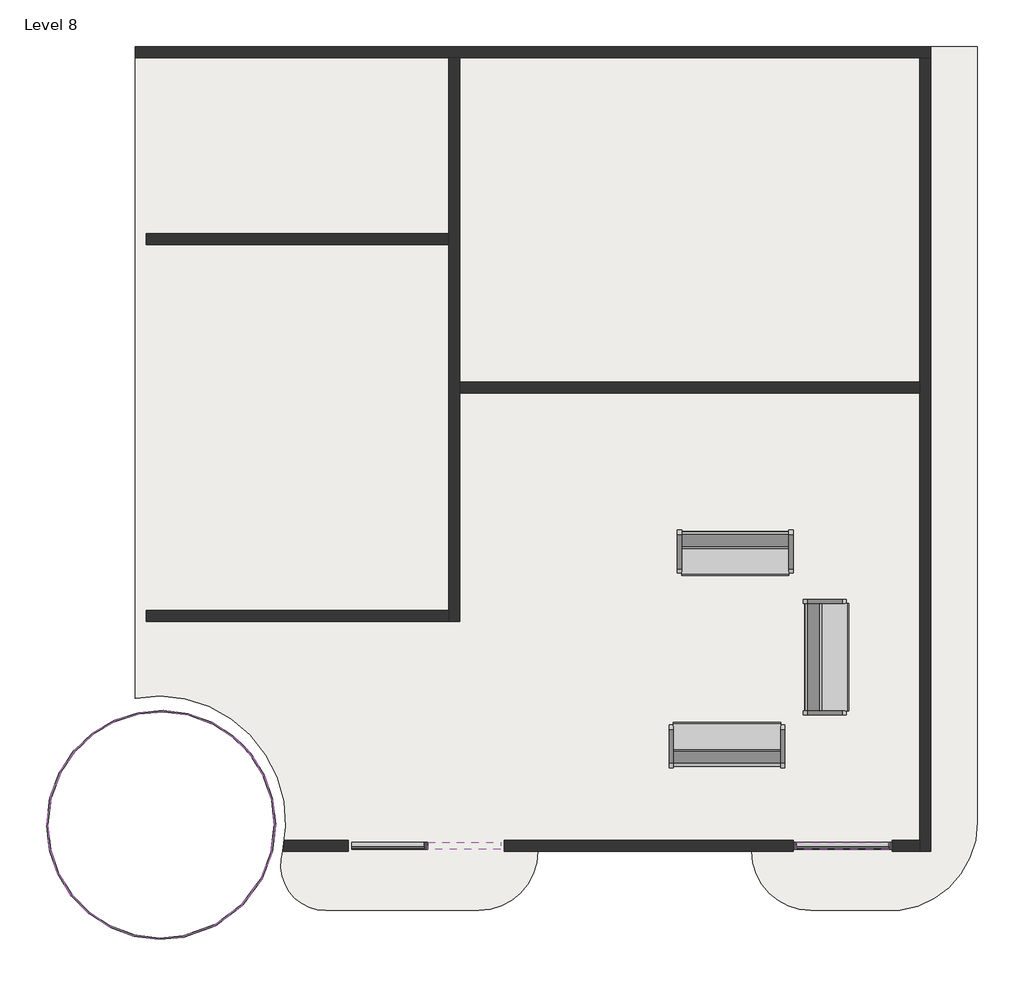
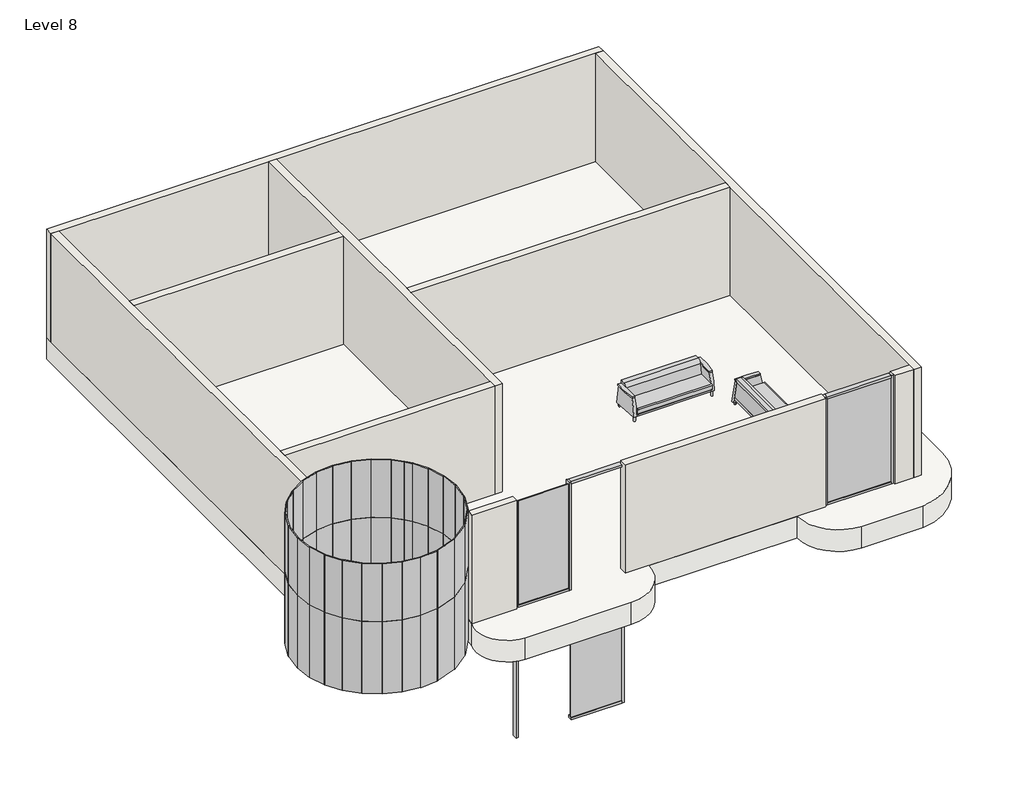
# One storey, incomplete: 59 plates, 11 members, 10 walls, 3 furniture elements, 1 slab.
"""IFC4 building model written with IfcOpenShell, lengths in millimetres."""

from ifc_helpers import new_model, si_unit, point, frame, frame_2d, origin, place, context, project, spatial, polyline, circle_curve, trimmed, segment, composite_curve, outline, extrude, faceted_brep, transform, mapped, element, save
from ifc_brep_helpers import plane_surface, revolved_surface, advanced_brep
from components import furniture_aff9b2fb, member_eaba9652, member_3f395ae9, member_0c868e12, member_7bc42366, system_panel_glazed_f1c144f9, system_panel_glazed_8ed2b2ee, system_panel_glazed_c7815b78, system_panel_glazed_220ba5f3, system_panel_glazed_11fb153e, system_panel_glazed_2f540b85, system_panel_glazed_4848e608, system_panel_glazed_8b35a0ff, system_panel_glazed_87282c25, system_panel_glazed_6d1bb68c, system_panel_glazed_cb3ffd69, system_panel_glazed_404d015f, system_panel_glazed_7b556abe, system_panel_glazed_370bf902

model = new_model("IFC4")

# Units and contexts
model_context = context("Model", 3, world=origin())
ifc_project = project(units=[si_unit("LENGTHUNIT", "METRE", prefix="MILLI")], contexts=[model_context])

# Site, building, storey
site = spatial("IfcSite", under=ifc_project)
building = spatial("IfcBuilding", under=site)
storey = spatial("IfcBuildingStorey", under=building, Name="Level 8", Elevation=21336.0)

# Furniture
placement = place(None, origin())
furniture_shape = furniture_aff9b2fb(model_context)
element("IfcFurniture", 1, ObjectType="Sofa-Pensi : 84\"", at=placement, inside=storey, context=model_context, shape_type="MappedRepresentation", body=[
    mapped(furniture_shape, transform((-2244.8524991, 3650.1964615, 21945.6), x_axis=(1.0, 0.0, 0.0), y_axis=(0.0, 1.0, 0.0), z_axis=(0.0, 0.0, 1.0))),
])
element("IfcFurniture", 2, ObjectType="Sofa-Pensi : 84\"", at=placement, inside=storey, context=model_context, shape_type="MappedRepresentation", body=[
    mapped(furniture_shape, transform((-12.736413, 1720.492712, 21945.6), x_axis=(0.0, 1.0, 0.0), y_axis=(-1.0, 0.0, 0.0), z_axis=(0.0, 0.0, 1.0))),
])
element("IfcFurniture", 3, ObjectType="Sofa-Pensi : 84\"", at=placement, inside=storey, context=model_context, shape_type="MappedRepresentation", body=[
    mapped(furniture_shape, transform((-1840.0399991, 648.4161336, 21945.6), x_axis=(-1.0, 0.0, 0.0), y_axis=(0.0, -1.0, 0.0), z_axis=(0.0, 0.0, 1.0))),
])

# Members
member_shape = member_eaba9652(model_context)
element("IfcMember", 4, ObjectType="Rectangular Mullion : 2.5\" x 5\" rectangular", at=placement, inside=storey, context=model_context, shape_type="MappedRepresentation", body=[
    mapped(member_shape, transform((-7672.5789001, -1482.8937024, 21945.6), x_axis=(-1.0, 0.0, 0.0), y_axis=(0.0, 1.0, 0.0), z_axis=(0.0, 0.0, -1.0))),
])
member_2_shape = member_3f395ae9(model_context)
element("IfcMember", 5, ObjectType="Rectangular Mullion : 2.5\" x 5\" rectangular", at=placement, inside=storey, context=model_context, shape_type="MappedRepresentation", body=[
    mapped(member_2_shape, transform((-9111.7115512, -1482.8937024, 18288.0), x_axis=(-1.0, 0.0, 0.0), y_axis=(0.0, 1.0, 0.0), z_axis=(0.0, 0.0, -1.0))),
])
element("IfcMember", 6, ObjectType="Rectangular Mullion : 2.5\" x 5\" rectangular", at=placement, inside=storey, context=model_context, shape_type="MappedRepresentation", body=[
    mapped(member_2_shape, transform((-899.4462491, -1482.8937024, 21945.6), x_axis=(-1.0, 0.0, 0.0), y_axis=(0.0, 1.0, 0.0), z_axis=(0.0, 0.0, -1.0))),
])
element("IfcMember", 7, ObjectType="Rectangular Mullion : 2.5\" x 5\" rectangular", at=placement, inside=storey, context=model_context, shape_type="MappedRepresentation", body=[
    mapped(member_2_shape, transform((-6233.4462491, -1482.8937024, 21336.0), x_axis=(1.0, 0.0, 0.0), y_axis=(0.0, 1.0, 0.0), z_axis=(0.0, 0.0, 1.0))),
])
element("IfcMember", 8, ObjectType="Rectangular Mullion : 2.5\" x 5\" rectangular", at=placement, inside=storey, context=model_context, shape_type="MappedRepresentation", body=[
    mapped(member_2_shape, transform((929.3537509, -1482.8937024, 24993.6), x_axis=(1.0, 0.0, 0.0), y_axis=(0.0, 1.0, 0.0), z_axis=(0.0, 0.0, 1.0))),
])
member_3_shape = member_0c868e12(model_context)
element("IfcMember", 9, ObjectType="Rectangular Mullion : 2.5\" x 5\" rectangular", at=placement, inside=storey, context=model_context, shape_type="MappedRepresentation", body=[
    mapped(member_3_shape, transform((-9048.2115512, -1482.8937024, 21336.0), x_axis=(0.0, 0.0, 1.0), y_axis=(0.0, 1.0, 0.0), z_axis=(-1.0, 0.0, 0.0))),
])
element("IfcMember", 10, ObjectType="Rectangular Mullion : 2.5\" x 5\" rectangular", at=placement, inside=storey, context=model_context, shape_type="MappedRepresentation", body=[
    mapped(member_3_shape, transform((-7640.8289001, -1482.8937024, 24993.6), x_axis=(0.0, 0.0, 1.0), y_axis=(0.0, 1.0, 0.0), z_axis=(-1.0, 0.0, 0.0))),
])
element("IfcMember", 11, ObjectType="Rectangular Mullion : 2.5\" x 5\" rectangular", at=placement, inside=storey, context=model_context, shape_type="MappedRepresentation", body=[
    mapped(member_3_shape, transform((-6296.9462491, -1482.8937024, 18288.0), x_axis=(0.0, 0.0, -1.0), y_axis=(0.0, 1.0, 0.0), z_axis=(1.0, 0.0, 0.0))),
])
element("IfcMember", 12, ObjectType="Rectangular Mullion : 2.5\" x 5\" rectangular", at=placement, inside=storey, context=model_context, shape_type="MappedRepresentation", body=[
    mapped(member_3_shape, transform((-7704.3289001, -1482.8937024, 21945.6), x_axis=(0.0, 0.0, -1.0), y_axis=(0.0, 1.0, 0.0), z_axis=(1.0, 0.0, 0.0))),
])
member_4_shape = member_7bc42366(model_context)
element("IfcMember", 13, ObjectType="Rectangular Mullion : 2.5\" x 5\" rectangular", at=placement, inside=storey, context=model_context, shape_type="MappedRepresentation", body=[
    mapped(member_4_shape, transform((-835.9462491, -1482.8937024, 24993.6), x_axis=(0.0, 0.0, 1.0), y_axis=(0.0, 1.0, 0.0), z_axis=(-1.0, 0.0, 0.0))),
])
element("IfcMember", 14, ObjectType="Rectangular Mullion : 2.5\" x 5\" rectangular", at=placement, inside=storey, context=model_context, shape_type="MappedRepresentation", body=[
    mapped(member_4_shape, transform((865.8537509, -1482.8937024, 21945.6), x_axis=(0.0, 0.0, -1.0), y_axis=(0.0, 1.0, 0.0), z_axis=(1.0, 0.0, 0.0))),
])

# Plates
system_panel_glazed_shape = system_panel_glazed_f1c144f9(model_context)
element("IfcPlate", 15, ObjectType="System Panel : Glazed", at=placement, inside=storey, context=model_context, shape_type="MappedRepresentation", body=[
    mapped(system_panel_glazed_shape, transform((-14541.9245022, -346.5978939, 21945.6), x_axis=(-0.3551689475306269, -0.9348021281051873, 0.0), y_axis=(0.9348021281051873, -0.3551689475306269, 0.0), z_axis=(0.0, 0.0, 1.0))),
])
element("IfcPlate", 16, ObjectType="System Panel : Glazed", at=placement, inside=storey, context=model_context, shape_type="MappedRepresentation", body=[
    mapped(system_panel_glazed_shape, transform((-10582.1178502, -1851.0877948, 21945.6), x_axis=(0.35516894753064066, 0.934802128105182, 0.0), y_axis=(-0.934802128105182, 0.35516894753064066, 0.0), z_axis=(0.0, 0.0, 1.0))),
])
element("IfcPlate", 17, ObjectType="System Panel : Glazed", at=placement, inside=storey, context=model_context, shape_type="MappedRepresentation", body=[
    mapped(system_panel_glazed_shape, transform((-10459.5232171, -1354.5613954, 21945.6), x_axis=(0.12073632210407237, 0.9926846128175765, 0.0), y_axis=(-0.9926846128175765, 0.12073632210407237, 0.0), z_axis=(0.0, 0.0, 1.0))),
])
element("IfcPlate", 18, ObjectType="System Panel : Glazed", at=placement, inside=storey, context=model_context, shape_type="MappedRepresentation", body=[
    mapped(system_panel_glazed_shape, transform((-14664.5191354, -843.1242933, 21945.6), x_axis=(-0.12073632210406239, -0.9926846128175777, 0.0), y_axis=(0.9926846128175777, -0.12073632210406239, 0.0), z_axis=(0.0, 0.0, 1.0))),
])
system_panel_glazed_2_shape = system_panel_glazed_8ed2b2ee(model_context)
element("IfcPlate", 19, ObjectType="System Panel : Glazed", at=placement, inside=storey, context=model_context, shape_type="MappedRepresentation", body=[
    mapped(system_panel_glazed_2_shape, transform((-11841.3777431, -3082.3793017, 21945.6), x_axis=(0.9398911711666007, 0.3414741371803665, 0.0), y_axis=(-0.3414741371803665, 0.9398911711666007, 0.0), z_axis=(0.0, 0.0, 1.0))),
])
element("IfcPlate", 20, ObjectType="System Panel : Glazed", at=placement, inside=storey, context=model_context, shape_type="MappedRepresentation", body=[
    mapped(system_panel_glazed_2_shape, transform((-10858.9635423, -2345.1728692, 21945.6), x_axis=(0.5905687200141164, 0.8069873524045393, 0.0), y_axis=(-0.8069873524045393, 0.5905687200141164, 0.0), z_axis=(0.0, 0.0, 1.0))),
])
element("IfcPlate", 21, ObjectType="System Panel : Glazed", at=placement, inside=storey, context=model_context, shape_type="MappedRepresentation", body=[
    mapped(system_panel_glazed_2_shape, transform((-11295.3522982, -2786.8279712, 21945.6), x_axis=(0.7998453025525061, 0.6002062078858317, 0.0), y_axis=(-0.6002062078858317, 0.7998453025525061, 0.0), z_axis=(0.0, 0.0, 1.0))),
])
system_panel_glazed_3_shape = system_panel_glazed_c7815b78(model_context)
element("IfcPlate", 22, ObjectType="System Panel : Glazed", at=placement, inside=storey, context=model_context, shape_type="MappedRepresentation", body=[
    mapped(system_panel_glazed_3_shape, transform((-10454.4737362, -864.5204039, 21945.6), x_axis=(-0.11050163420416614, 0.993875942378227, 0.0), y_axis=(-0.993875942378227, -0.11050163420416614, 0.0), z_axis=(0.0, 0.0, 1.0))),
])
element("IfcPlate", 23, ObjectType="System Panel : Glazed", at=placement, inside=storey, context=model_context, shape_type="MappedRepresentation", body=[
    mapped(system_panel_glazed_3_shape, transform((-14669.5686163, -1333.1652848, 21945.6), x_axis=(0.11050163420415136, -0.9938759423782286, 0.0), y_axis=(0.9938759423782286, 0.11050163420415136, 0.0), z_axis=(0.0, 0.0, 1.0))),
])
element("IfcPlate", 24, ObjectType="System Panel : Glazed", at=placement, inside=storey, context=model_context, shape_type="MappedRepresentation", body=[
    mapped(system_panel_glazed_3_shape, transform((-11410.1424167, 681.5611944, 21945.6), x_axis=(-0.8396018558176894, 0.5432022861766066, 0.0), y_axis=(-0.5432022861766066, -0.8396018558176894, 0.0), z_axis=(0.0, 0.0, 1.0))),
])
element("IfcPlate", 25, ObjectType="System Panel : Glazed", at=placement, inside=storey, context=model_context, shape_type="MappedRepresentation", body=[
    mapped(system_panel_glazed_3_shape, transform((-13212.0893695, 919.590846, 21945.6), x_axis=(-0.9518517343814786, -0.3065587639506839, 0.0), y_axis=(0.3065587639506839, -0.9518517343814786, 0.0), z_axis=(0.0, 0.0, 1.0))),
])
element("IfcPlate", 26, ObjectType="System Panel : Glazed", at=placement, inside=storey, context=model_context, shape_type="MappedRepresentation", body=[
    mapped(system_panel_glazed_3_shape, transform((-12839.7224363, -3201.1142893, 21945.6), x_axis=(0.9913878918151698, -0.1309581916577702, 0.0), y_axis=(0.1309581916577702, 0.9913878918151698, 0.0), z_axis=(0.0, 0.0, 1.0))),
])
element("IfcPlate", 27, ObjectType="System Panel : Glazed", at=placement, inside=storey, context=model_context, shape_type="MappedRepresentation", body=[
    mapped(system_panel_glazed_3_shape, transform((-14365.783041, -2213.7896382, 21945.6), x_axis=(0.5257859322352114, -0.8506169252157811, 0.0), y_axis=(0.8506169252157811, 0.5257859322352114, 0.0), z_axis=(0.0, 0.0, 1.0))),
])
element("IfcPlate", 28, ObjectType="System Panel : Glazed", at=placement, inside=storey, context=model_context, shape_type="MappedRepresentation", body=[
    mapped(system_panel_glazed_3_shape, transform((-13713.8999358, -2879.2468831, 21945.6), x_axis=(0.8396018558176805, -0.5432022861766201, 0.0), y_axis=(0.5432022861766201, 0.8396018558176805, 0.0), z_axis=(0.0, 0.0, 1.0))),
])
element("IfcPlate", 29, ObjectType="System Panel : Glazed", at=placement, inside=storey, context=model_context, shape_type="MappedRepresentation", body=[
    mapped(system_panel_glazed_3_shape, transform((-14014.4059364, 446.2272921, 21945.6), x_axis=(-0.7286232370002992, -0.6849147235263715, 0.0), y_axis=(0.6849147235263715, -0.7286232370002992, 0.0), z_axis=(0.0, 0.0, 1.0))),
])
element("IfcPlate", 30, ObjectType="System Panel : Glazed", at=placement, inside=storey, context=model_context, shape_type="MappedRepresentation", body=[
    mapped(system_panel_glazed_3_shape, transform((-12284.3199161, 1003.4286006, 21945.6), x_axis=(-0.9913878918151723, 0.13095819165775144, 0.0), y_axis=(-0.13095819165775144, -0.9913878918151723, 0.0), z_axis=(0.0, 0.0, 1.0))),
])
element("IfcPlate", 31, ObjectType="System Panel : Glazed", at=placement, inside=storey, context=model_context, shape_type="MappedRepresentation", body=[
    mapped(system_panel_glazed_3_shape, transform((-12752.8652893, 1013.0855973, 21945.6), x_axis=(-0.9959419324521102, -0.08999815100076568, 0.0), y_axis=(0.08999815100076568, -0.9959419324521102, 0.0), z_axis=(0.0, 0.0, 1.0))),
])
element("IfcPlate", 32, ObjectType="System Panel : Glazed", at=placement, inside=storey, context=model_context, shape_type="MappedRepresentation", body=[
    mapped(system_panel_glazed_3_shape, transform((-11829.3381514, 891.0915272, 21945.6), x_axis=(-0.9384120429483949, 0.3455182160891376, 0.0), y_axis=(-0.3455182160891376, -0.9384120429483949, 0.0), z_axis=(0.0, 0.0, 1.0))),
])
element("IfcPlate", 33, ObjectType="System Panel : Glazed", at=placement, inside=storey, context=model_context, shape_type="MappedRepresentation", body=[
    mapped(system_panel_glazed_3_shape, transform((-10557.4115054, -407.3204039, 21945.6), x_axis=(-0.3261077326604367, 0.9453326116764772, 0.0), y_axis=(-0.9453326116764772, -0.3261077326604367, 0.0), z_axis=(0.0, 0.0, 1.0))),
])
element("IfcPlate", 34, ObjectType="System Panel : Glazed", at=placement, inside=storey, context=model_context, shape_type="MappedRepresentation", body=[
    mapped(system_panel_glazed_3_shape, transform((-12371.1770631, -3210.771286, 21945.6), x_axis=(0.9959419324521115, 0.08999815100075001, 0.0), y_axis=(-0.08999815100075001, 0.9959419324521115, 0.0), z_axis=(0.0, 0.0, 1.0))),
])
element("IfcPlate", 35, ObjectType="System Panel : Glazed", at=placement, inside=storey, context=model_context, shape_type="MappedRepresentation", body=[
    mapped(system_panel_glazed_3_shape, transform((-13294.7042011, -3088.7772159, 21945.6), x_axis=(0.9384120429483891, -0.34551821608915334, 0.0), y_axis=(0.34551821608915334, 0.9384120429483891, 0.0), z_axis=(0.0, 0.0, 1.0))),
])
element("IfcPlate", 36, ObjectType="System Panel : Glazed", at=placement, inside=storey, context=model_context, shape_type="MappedRepresentation", body=[
    mapped(system_panel_glazed_3_shape, transform((-14076.8350959, -2582.7572647, 21945.6), x_axis=(0.6997834615185511, -0.7143550286692988, 0.0), y_axis=(0.7143550286692988, 0.6997834615185511, 0.0), z_axis=(0.0, 0.0, 1.0))),
])
element("IfcPlate", 37, ObjectType="System Panel : Glazed", at=placement, inside=storey, context=model_context, shape_type="MappedRepresentation", body=[
    mapped(system_panel_glazed_3_shape, transform((-14566.6308471, -1790.3652848, 21945.6), x_axis=(0.32610773266042153, -0.9453326116764824, 0.0), y_axis=(0.9453326116764824, 0.32610773266042153, 0.0), z_axis=(0.0, 0.0, 1.0))),
])
element("IfcPlate", 38, ObjectType="System Panel : Glazed", at=placement, inside=storey, context=model_context, shape_type="MappedRepresentation", body=[
    mapped(system_panel_glazed_3_shape, transform((-14318.3113206, 89.4787227, 21945.6), x_axis=(-0.5603879632167612, -0.8282302401396425, 0.0), y_axis=(0.8282302401396425, -0.5603879632167612, 0.0), z_axis=(0.0, 0.0, 1.0))),
])
element("IfcPlate", 39, ObjectType="System Panel : Glazed", at=placement, inside=storey, context=model_context, shape_type="MappedRepresentation", body=[
    mapped(system_panel_glazed_3_shape, transform((-13639.5625299, 727.5108588, 21945.6), x_axis=(-0.8612707706620224, -0.5081462974412448, 0.0), y_axis=(0.5081462974412448, -0.8612707706620224, 0.0), z_axis=(0.0, 0.0, 1.0))),
])
system_panel_glazed_4_shape = system_panel_glazed_220ba5f3(model_context)
element("IfcPlate", 40, ObjectType="System Panel : Glazed", at=placement, inside=storey, context=model_context, shape_type="MappedRepresentation", body=[
    mapped(system_panel_glazed_4_shape, transform((-10742.3305673, -4.7597883, 21945.6), x_axis=(-0.5152811917631037, 0.8570211744263939, 0.0), y_axis=(-0.8570211744263939, -0.5152811917631037, 0.0), z_axis=(0.0, 0.0, 1.0))),
])
system_panel_glazed_5_shape = system_panel_glazed_11fb153e(model_context)
element("IfcPlate", 41, ObjectType="System Panel : Glazed", at=placement, inside=storey, context=model_context, shape_type="MappedRepresentation", body=[
    mapped(system_panel_glazed_5_shape, transform((-11098.0043985, 445.2241463, 21945.6), x_axis=(-0.7256671855033587, 0.6880458821064435, 0.0), y_axis=(-0.6880458821064435, -0.7256671855033587, 0.0), z_axis=(0.0, 0.0, 1.0))),
])
system_panel_glazed_6_shape = system_panel_glazed_2f540b85(model_context)
element("IfcPlate", 42, ObjectType="System Panel : Glazed", at=placement, inside=storey, context=model_context, shape_type="MappedRepresentation", body=[
    mapped(system_panel_glazed_6_shape, transform((-10917.0903061, 255.9395759, 21945.6), x_axis=(-0.6357445726375757, 0.7718995001694627, 0.0), y_axis=(-0.7718995001694627, -0.6357445726375757, 0.0), z_axis=(0.0, 0.0, 1.0))),
])
system_panel_glazed_7_shape = system_panel_glazed_4848e608(model_context)
element("IfcPlate", 43, ObjectType="System Panel : Glazed", at=placement, inside=storey, context=model_context, shape_type="MappedRepresentation", body=[
    mapped(system_panel_glazed_7_shape, transform((-14669.5686163, -1333.1652848, 23977.6), x_axis=(0.11050163420415136, -0.9938759423782286, 0.0), y_axis=(0.9938759423782286, 0.11050163420415136, 0.0), z_axis=(0.0, 0.0, 1.0))),
])
element("IfcPlate", 44, ObjectType="System Panel : Glazed", at=placement, inside=storey, context=model_context, shape_type="MappedRepresentation", body=[
    mapped(system_panel_glazed_7_shape, transform((-14365.783041, -2213.7896382, 23977.6), x_axis=(0.5257859322352114, -0.8506169252157811, 0.0), y_axis=(0.8506169252157811, 0.5257859322352114, 0.0), z_axis=(0.0, 0.0, 1.0))),
])
element("IfcPlate", 45, ObjectType="System Panel : Glazed", at=placement, inside=storey, context=model_context, shape_type="MappedRepresentation", body=[
    mapped(system_panel_glazed_7_shape, transform((-13713.8999358, -2879.2468831, 23977.6), x_axis=(0.8396018558176805, -0.5432022861766201, 0.0), y_axis=(0.5432022861766201, 0.8396018558176805, 0.0), z_axis=(0.0, 0.0, 1.0))),
])
element("IfcPlate", 46, ObjectType="System Panel : Glazed", at=placement, inside=storey, context=model_context, shape_type="MappedRepresentation", body=[
    mapped(system_panel_glazed_7_shape, transform((-12839.7224363, -3201.1142893, 23977.6), x_axis=(0.9913878918151698, -0.13095819165777017, 0.0), y_axis=(0.13095819165777017, 0.9913878918151698, 0.0), z_axis=(0.0, 0.0, 1.0))),
])
element("IfcPlate", 47, ObjectType="System Panel : Glazed", at=placement, inside=storey, context=model_context, shape_type="MappedRepresentation", body=[
    mapped(system_panel_glazed_7_shape, transform((-12371.1770631, -3210.771286, 23977.6), x_axis=(0.9959419324521115, 0.08999815100075001, 0.0), y_axis=(-0.08999815100075001, 0.9959419324521115, 0.0), z_axis=(0.0, 0.0, 1.0))),
])
element("IfcPlate", 48, ObjectType="System Panel : Glazed", at=placement, inside=storey, context=model_context, shape_type="MappedRepresentation", body=[
    mapped(system_panel_glazed_7_shape, transform((-13294.7042011, -3088.7772159, 23977.6), x_axis=(0.9384120429483891, -0.34551821608915334, 0.0), y_axis=(0.34551821608915334, 0.9384120429483891, 0.0), z_axis=(0.0, 0.0, 1.0))),
])
element("IfcPlate", 49, ObjectType="System Panel : Glazed", at=placement, inside=storey, context=model_context, shape_type="MappedRepresentation", body=[
    mapped(system_panel_glazed_7_shape, transform((-14076.8350959, -2582.7572647, 23977.6), x_axis=(0.6997834615185511, -0.7143550286692988, 0.0), y_axis=(0.7143550286692988, 0.6997834615185511, 0.0), z_axis=(0.0, 0.0, 1.0))),
])
element("IfcPlate", 50, ObjectType="System Panel : Glazed", at=placement, inside=storey, context=model_context, shape_type="MappedRepresentation", body=[
    mapped(system_panel_glazed_7_shape, transform((-14566.6308471, -1790.3652848, 23977.6), x_axis=(0.32610773266042153, -0.9453326116764824, 0.0), y_axis=(0.9453326116764824, 0.32610773266042153, 0.0), z_axis=(0.0, 0.0, 1.0))),
])
element("IfcPlate", 51, ObjectType="System Panel : Glazed", at=placement, inside=storey, context=model_context, shape_type="MappedRepresentation", body=[
    mapped(system_panel_glazed_7_shape, transform((-10454.4737362, -864.5204039, 23977.6), x_axis=(-0.11050163420416614, 0.993875942378227, 0.0), y_axis=(-0.993875942378227, -0.11050163420416614, 0.0), z_axis=(0.0, 0.0, 1.0))),
])
element("IfcPlate", 52, ObjectType="System Panel : Glazed", at=placement, inside=storey, context=model_context, shape_type="MappedRepresentation", body=[
    mapped(system_panel_glazed_7_shape, transform((-10557.4115054, -407.3204039, 23977.6), x_axis=(-0.3261077326604368, 0.9453326116764772, 0.0), y_axis=(-0.9453326116764772, -0.3261077326604368, 0.0), z_axis=(0.0, 0.0, 1.0))),
])
element("IfcPlate", 53, ObjectType="System Panel : Glazed", at=placement, inside=storey, context=model_context, shape_type="MappedRepresentation", body=[
    mapped(system_panel_glazed_7_shape, transform((-11410.1424167, 681.5611944, 23977.6), x_axis=(-0.8396018558176894, 0.5432022861766066, 0.0), y_axis=(-0.5432022861766066, -0.8396018558176894, 0.0), z_axis=(0.0, 0.0, 1.0))),
])
element("IfcPlate", 54, ObjectType="System Panel : Glazed", at=placement, inside=storey, context=model_context, shape_type="MappedRepresentation", body=[
    mapped(system_panel_glazed_7_shape, transform((-11829.3381514, 891.0915272, 23977.6), x_axis=(-0.9384120429483949, 0.3455182160891376, 0.0), y_axis=(-0.3455182160891376, -0.9384120429483949, 0.0), z_axis=(0.0, 0.0, 1.0))),
])
element("IfcPlate", 55, ObjectType="System Panel : Glazed", at=placement, inside=storey, context=model_context, shape_type="MappedRepresentation", body=[
    mapped(system_panel_glazed_7_shape, transform((-12284.3199161, 1003.4286006, 23977.6), x_axis=(-0.9913878918151723, 0.1309581916577514, 0.0), y_axis=(-0.1309581916577514, -0.9913878918151723, 0.0), z_axis=(0.0, 0.0, 1.0))),
])
element("IfcPlate", 56, ObjectType="System Panel : Glazed", at=placement, inside=storey, context=model_context, shape_type="MappedRepresentation", body=[
    mapped(system_panel_glazed_7_shape, transform((-12752.8652893, 1013.0855973, 23977.6), x_axis=(-0.9959419324521102, -0.08999815100076568, 0.0), y_axis=(0.08999815100076568, -0.9959419324521102, 0.0), z_axis=(0.0, 0.0, 1.0))),
])
element("IfcPlate", 57, ObjectType="System Panel : Glazed", at=placement, inside=storey, context=model_context, shape_type="MappedRepresentation", body=[
    mapped(system_panel_glazed_7_shape, transform((-13212.0893695, 919.590846, 23977.6), x_axis=(-0.9518517343814786, -0.3065587639506839, 0.0), y_axis=(0.3065587639506839, -0.9518517343814786, 0.0), z_axis=(0.0, 0.0, 1.0))),
])
element("IfcPlate", 58, ObjectType="System Panel : Glazed", at=placement, inside=storey, context=model_context, shape_type="MappedRepresentation", body=[
    mapped(system_panel_glazed_7_shape, transform((-13639.5625299, 727.5108588, 23977.6), x_axis=(-0.8612707706620223, -0.508146297441245, 0.0), y_axis=(0.508146297441245, -0.8612707706620223, 0.0), z_axis=(0.0, 0.0, 1.0))),
])
element("IfcPlate", 59, ObjectType="System Panel : Glazed", at=placement, inside=storey, context=model_context, shape_type="MappedRepresentation", body=[
    mapped(system_panel_glazed_7_shape, transform((-14014.4059364, 446.2272921, 23977.6), x_axis=(-0.7286232370002992, -0.6849147235263715, 0.0), y_axis=(0.6849147235263715, -0.7286232370002992, 0.0), z_axis=(0.0, 0.0, 1.0))),
])
element("IfcPlate", 60, ObjectType="System Panel : Glazed", at=placement, inside=storey, context=model_context, shape_type="MappedRepresentation", body=[
    mapped(system_panel_glazed_7_shape, transform((-14318.3113206, 89.4787227, 23977.6), x_axis=(-0.5603879632167612, -0.8282302401396425, 0.0), y_axis=(0.8282302401396425, -0.5603879632167612, 0.0), z_axis=(0.0, 0.0, 1.0))),
])
system_panel_glazed_8_shape = system_panel_glazed_8b35a0ff(model_context)
element("IfcPlate", 61, ObjectType="System Panel : Glazed", at=placement, inside=storey, context=model_context, shape_type="MappedRepresentation", body=[
    mapped(system_panel_glazed_8_shape, transform((-10742.3305673, -4.7597883, 23977.6), x_axis=(-0.5152811917631037, 0.8570211744263939, 0.0), y_axis=(-0.8570211744263939, -0.5152811917631037, 0.0), z_axis=(0.0, 0.0, 1.0))),
])
system_panel_glazed_9_shape = system_panel_glazed_87282c25(model_context)
element("IfcPlate", 62, ObjectType="System Panel : Glazed", at=placement, inside=storey, context=model_context, shape_type="MappedRepresentation", body=[
    mapped(system_panel_glazed_9_shape, transform((-10917.0903061, 255.9395759, 23977.6), x_axis=(-0.6357445726375757, 0.7718995001694627, 0.0), y_axis=(-0.7718995001694627, -0.6357445726375757, 0.0), z_axis=(0.0, 0.0, 1.0))),
])
system_panel_glazed_10_shape = system_panel_glazed_6d1bb68c(model_context)
element("IfcPlate", 63, ObjectType="System Panel : Glazed", at=placement, inside=storey, context=model_context, shape_type="MappedRepresentation", body=[
    mapped(system_panel_glazed_10_shape, transform((-11098.0043985, 445.2241463, 23977.6), x_axis=(-0.7256671855033587, 0.6880458821064435, 0.0), y_axis=(-0.6880458821064435, -0.7256671855033587, 0.0), z_axis=(0.0, 0.0, 1.0))),
])
system_panel_glazed_11_shape = system_panel_glazed_cb3ffd69(model_context)
element("IfcPlate", 64, ObjectType="System Panel : Glazed", at=placement, inside=storey, context=model_context, shape_type="MappedRepresentation", body=[
    mapped(system_panel_glazed_11_shape, transform((-10582.1178502, -1851.0877948, 23977.6), x_axis=(0.35516894753064066, 0.934802128105182, 0.0), y_axis=(-0.934802128105182, 0.35516894753064066, 0.0), z_axis=(0.0, 0.0, 1.0))),
])
element("IfcPlate", 65, ObjectType="System Panel : Glazed", at=placement, inside=storey, context=model_context, shape_type="MappedRepresentation", body=[
    mapped(system_panel_glazed_11_shape, transform((-10459.5232171, -1354.5613954, 23977.6), x_axis=(0.1207363221040724, 0.9926846128175765, 0.0), y_axis=(-0.9926846128175765, 0.1207363221040724, 0.0), z_axis=(0.0, 0.0, 1.0))),
])
element("IfcPlate", 66, ObjectType="System Panel : Glazed", at=placement, inside=storey, context=model_context, shape_type="MappedRepresentation", body=[
    mapped(system_panel_glazed_11_shape, transform((-14541.9245022, -346.5978939, 23977.6), x_axis=(-0.3551689475306269, -0.9348021281051873, 0.0), y_axis=(0.9348021281051873, -0.3551689475306269, 0.0), z_axis=(0.0, 0.0, 1.0))),
])
element("IfcPlate", 67, ObjectType="System Panel : Glazed", at=placement, inside=storey, context=model_context, shape_type="MappedRepresentation", body=[
    mapped(system_panel_glazed_11_shape, transform((-14664.5191354, -843.1242933, 23977.6), x_axis=(-0.1207363221040624, -0.9926846128175777, 0.0), y_axis=(0.9926846128175777, -0.1207363221040624, 0.0), z_axis=(0.0, 0.0, 1.0))),
])
system_panel_glazed_12_shape = system_panel_glazed_404d015f(model_context)
element("IfcPlate", 68, ObjectType="System Panel : Glazed", at=placement, inside=storey, context=model_context, shape_type="MappedRepresentation", body=[
    mapped(system_panel_glazed_12_shape, transform((-11841.3777431, -3082.3793017, 23977.6), x_axis=(0.9398911711666007, 0.3414741371803665, 0.0), y_axis=(-0.3414741371803665, 0.9398911711666007, 0.0), z_axis=(0.0, 0.0, 1.0))),
])
element("IfcPlate", 69, ObjectType="System Panel : Glazed", at=placement, inside=storey, context=model_context, shape_type="MappedRepresentation", body=[
    mapped(system_panel_glazed_12_shape, transform((-10858.9635423, -2345.1728692, 23977.6), x_axis=(0.5905687200141164, 0.8069873524045393, 0.0), y_axis=(-0.8069873524045393, 0.5905687200141164, 0.0), z_axis=(0.0, 0.0, 1.0))),
])
element("IfcPlate", 70, ObjectType="System Panel : Glazed", at=placement, inside=storey, context=model_context, shape_type="MappedRepresentation", body=[
    mapped(system_panel_glazed_12_shape, transform((-11295.3522982, -2786.8279712, 23977.6), x_axis=(0.7998453025525062, 0.6002062078858316, 0.0), y_axis=(-0.6002062078858316, 0.7998453025525062, 0.0), z_axis=(0.0, 0.0, 1.0))),
])
system_panel_glazed_13_shape = system_panel_glazed_7b556abe(model_context)
element("IfcPlate", 71, ObjectType="System Panel : Glazed", at=placement, inside=storey, context=model_context, shape_type="MappedRepresentation", body=[
    mapped(system_panel_glazed_13_shape, transform((-6968.8875746, -1482.8937024, 18351.5), x_axis=(-1.0, 0.0, 0.0), y_axis=(0.0, -1.0, 0.0), z_axis=(0.0, 0.0, 1.0))),
])
element("IfcPlate", 72, ObjectType="System Panel : Glazed", at=placement, inside=storey, context=model_context, shape_type="MappedRepresentation", body=[
    mapped(system_panel_glazed_13_shape, transform((-8376.2702257, -1482.8937024, 22009.1), x_axis=(-1.0, 0.0, 0.0), y_axis=(0.0, -1.0, 0.0), z_axis=(0.0, 0.0, 1.0))),
])
system_panel_glazed_14_shape = system_panel_glazed_370bf902(model_context)
element("IfcPlate", 73, ObjectType="System Panel : Glazed", at=placement, inside=storey, context=model_context, shape_type="MappedRepresentation", body=[
    mapped(system_panel_glazed_14_shape, transform((14.9537509, -1482.8937024, 22009.1), x_axis=(-1.0, 0.0, 0.0), y_axis=(0.0, -1.0, 0.0), z_axis=(0.0, 0.0, 1.0))),
])

# Slab
element("IfcSlab", 74, ObjectType="Generic - 2'", at=placement, inside=storey, context=model_context, shape_type="SweptSolid", body=[
    extrude(outline(composite_curve([segment(polyline([(2504.1537509, 13274.5062976), (2504.1537509, -1051.0937024)]), True, "CONTINUOUS"), segment(trimmed(circle_curve(frame_2d((865.9099456, -1051.0937024)), 1638.2438053), [point((2504.1537509, -1051.0937024))], [point((1069.0537509, -2676.6937024))], False, "CARTESIAN"), True, "CONTINUOUS"), segment(polyline([(1069.0537509, -2676.6937024), (-569.2462491, -2676.6937024)]), True, "CONTINUOUS"), segment(trimmed(circle_curve(frame_2d((-569.2462491, -1584.4937024)), 1092.2), [point((-569.2462491, -2676.6937024))], [point((-1661.4462491, -1584.4937024))], False, "CARTESIAN"), True, "CONTINUOUS"), segment(polyline([(-1661.4462491, -1584.4937024), (-5609.8647377, -1584.4937024)]), True, "CONTINUOUS"), segment(trimmed(circle_curve(frame_2d((-6702.0647377, -1584.4937024)), 1092.2), [point((-5609.8647377, -1584.4937024))], [point((-6702.0647377, -2676.6937024))], False, "CARTESIAN"), True, "CONTINUOUS"), segment(polyline([(-6702.0647377, -2676.6937024), (-9521.4647377, -2676.6937024)]), True, "CONTINUOUS"), segment(trimmed(circle_curve(frame_2d((-9521.4647377, -1843.8920375)), 832.801665), [point((-9521.4647377, -2676.6937024))], [point((-10312.8376694, -1584.4937024))], False, "CARTESIAN"), True, "CONTINUOUS"), segment(trimmed(circle_curve(frame_2d((-12612.6150686, -1075.1054509)), 2355.5153315), [point((-10312.8376694, -1584.4937024))], [point((-13040.6462491, 1241.1937063))], True, "CARTESIAN"), True, "CONTINUOUS"), segment(polyline([(-13040.6462491, 1241.1937063), (-13040.6462491, 13274.5062976), (2504.1537509, 13274.5062976)]), True, "CONTINUOUS")], self_intersect=False)), frame((0.0, 0.0, 21336.0), z_axis=(0.0, 0.0, 1.0), x_axis=(1.0, 0.0, 0.0)), (0.0, 0.0, 1.0), 609.6),
])

# Walls
element("IfcWall", 75, ObjectType="Generic - 8\"", at=placement, inside=storey, context=model_context, shape_type="Brep", body=[
    faceted_brep([(-13040.6462491, 13071.3062976, 21945.6), (-12837.4462491, 13071.3062976, 21945.6), (-7249.4462491, 13071.3062976, 21945.6), (-7046.2462491, 13071.3062976, 21945.6), (1437.3537509, 13071.3062976, 21945.6), (1640.5537509, 13071.3062976, 21945.6), (1640.5537509, 13071.3062976, 24993.6), (1437.3537509, 13071.3062976, 24993.6), (-7046.2462491, 13071.3062976, 24993.6), (-7249.4462491, 13071.3062976, 24993.6), (-12837.4462491, 13071.3062976, 24993.6), (-13040.6462491, 13071.3062976, 24993.6), (-13040.6462491, 13274.5062976, 21945.6), (-13040.6462491, 13274.5062976, 24993.6), (1640.5537509, 13274.5062976, 24993.6), (1640.5537509, 13274.5062976, 21945.6)], [[[0, 1, 2, 3, 4, 5, 6, 7, 8, 9, 10, 11]], [[12, 13, 14, 15]], [[5, 4, 3, 2, 1, 0, 12, 15]], [[11, 10, 9, 8, 7, 6, 14, 13]], [[6, 5, 15, 14]], [[0, 11, 13, 12]]]),
])
element("IfcWall", 76, ObjectType="Generic - 8\"", at=placement, inside=storey, context=model_context, shape_type="Brep", body=[
    faceted_brep([(1437.3537509, 13071.3062976, 21945.6), (1437.3537509, 7076.9062976, 21945.6), (1437.3537509, 6873.7062976, 21945.6), (1437.3537509, -1381.2937024, 21945.6), (1437.3537509, -1584.4937024, 21945.6), (1437.3537509, -1584.4937024, 24993.6), (1437.3537509, -1381.2937024, 24993.6), (1437.3537509, 6873.7062976, 24993.6), (1437.3537509, 7076.9062976, 24993.6), (1437.3537509, 13071.3062976, 24993.6), (1640.5537509, 13071.3062976, 21945.6), (1640.5537509, 13071.3062976, 24993.6), (1640.5537509, -1584.4937024, 24993.6), (1640.5537509, -1584.4937024, 21945.6)], [[[0, 1, 2, 3, 4, 5, 6, 7, 8, 9]], [[10, 11, 12, 13]], [[4, 3, 2, 1, 0, 10, 13]], [[9, 8, 7, 6, 5, 12, 11]], [[0, 9, 11, 10]], [[5, 4, 13, 12]]]),
])
element("IfcWall", 77, ObjectType="Generic - 8\"", at=placement, inside=storey, context=model_context, shape_type="AdvancedBrep", body=[
    advanced_brep(
    [(-13040.6462491, 13071.3062976, 21945.6), (-13040.6462491, 1241.1937063, 21945.6), (-13040.6462491, 1241.1937063, 24993.6), (-13040.6462491, 13071.3062976, 24993.6), (-12837.4462491, 13071.3062976, 21945.6), (-12837.4462491, 13071.3062976, 24993.6), (-12837.4462491, 9820.1062976, 24993.6), (-12837.4462491, 9616.9062976, 24993.6), (-12837.4462491, 2862.698962, 24993.6), (-12837.4462491, 2659.498962, 24993.6), (-12837.4462491, 1269.6553935, 24993.6), (-12837.4462491, 1269.6553935, 21945.6), (-12837.4462491, 2659.498962, 21945.6), (-12837.4462491, 2862.698962, 21945.6), (-12837.4462491, 9616.9062976, 21945.6), (-12837.4462491, 9820.1062976, 21945.6)],
    [
        (0, 1),
        (1, 2),
        (2, 3),
        (3, 0),
        (4, 5),
        (5, 6),
        (6, 7),
        (7, 8),
        (8, 9),
        (9, 10),
        (10, 11),
        (11, 12),
        (12, 13),
        (13, 14),
        (14, 15),
        (15, 4),
        (0, 4),
        (11, 1, circle_curve(frame((-12612.6150686, -1075.1054509, 21945.6), z_axis=(0.0, 0.0, 1.0), x_axis=(1.0, 0.0, 0.0)), 2355.5153315)),
        (2, 10, circle_curve(frame((-12612.6150686, -1075.1054509, 24993.6), z_axis=(0.0, 0.0, -1.0), x_axis=(1.0, 0.0, 0.0)), 2355.5153315)),
        (5, 3),
    ],
    [
        plane_surface(frame((-13040.6462491, 16068.5062976, 21945.6), z_axis=(-1.0, 0.0, 0.0), x_axis=(0.0, -1.0, 0.0))),
        plane_surface(frame((-12837.4462491, 16068.5062976, 21945.6), z_axis=(1.0, 0.0, 0.0), x_axis=(0.0, 1.0, 0.0))),
        plane_surface(frame((-13040.6462491, 13172.9062976, 21945.6), z_axis=(0.0, 0.0, -1.0), x_axis=(1.0, 0.0, 0.0))),
        plane_surface(frame((-13040.6462491, 1155.046339, 24993.6), z_axis=(0.0, 0.0, 1.0), x_axis=(1.0, 0.0, 0.0))),
        plane_surface(frame((-16139.4462491, 13071.3062976, 21945.6), z_axis=(0.0, 1.0, 0.0), x_axis=(1.0, 0.0, 0.0))),
        revolved_surface(polyline([(-10257.099737100001, -1075.1054509, 24993.6), (-10257.099737100001, -1075.1054509, 21945.6)]), (-12612.6150686, -1075.1054509, 21945.6), (0.0, 0.0, 1.0)),
    ],
    [
        (0, [[1, 2, 3, 4]]),
        (1, [[5, 6, 7, 8, 9, 10, 11, 12, 13, 14, 15, 16]]),
        (2, [[-1, 17, -16, -15, -14, -13, -12, 18]]),
        (3, [[-3, 19, -10, -9, -8, -7, -6, 20]]),
        (4, [[-4, -20, -5, -17]]),
        (5, [[-2, -18, -11, -19]]),
    ],
),
])
element("IfcWall", 78, ObjectType="Generic - 8\"", at=placement, inside=storey, context=model_context, shape_type="Brep", body=[
    faceted_brep([(-7249.4462491, 13071.3062976, 21945.6), (-7249.4462491, 9820.1062976, 21945.6), (-7249.4462491, 9616.9062976, 21945.6), (-7249.4462491, 2862.698962, 21945.6), (-7249.4462491, 2659.498962, 21945.6), (-7249.4462491, 2659.498962, 24993.6), (-7249.4462491, 2862.698962, 24993.6), (-7249.4462491, 9616.9062976, 24993.6), (-7249.4462491, 9820.1062976, 24993.6), (-7249.4462491, 13071.3062976, 24993.6), (-7046.2462491, 13071.3062976, 21945.6), (-7046.2462491, 13071.3062976, 24993.6), (-7046.2462491, 7076.9062976, 24993.6), (-7046.2462491, 6873.7062976, 24993.6), (-7046.2462491, 2659.498962, 24993.6), (-7046.2462491, 2659.498962, 21945.6), (-7046.2462491, 6873.7062976, 21945.6), (-7046.2462491, 7076.9062976, 21945.6)], [[[0, 1, 2, 3, 4, 5, 6, 7, 8, 9]], [[10, 11, 12, 13, 14, 15, 16, 17]], [[4, 3, 2, 1, 0, 10, 17, 16, 15]], [[9, 8, 7, 6, 5, 14, 13, 12, 11]], [[0, 9, 11, 10]], [[5, 4, 15, 14]]]),
])
element("IfcWall", 79, ObjectType="Generic - 8\"", at=placement, inside=storey, context=model_context, shape_type="SweptSolid", body=[
    extrude(outline(polyline([(1437.3537509, 6873.7062976), (-7046.2462491, 6873.7062976), (-7046.2462491, 7076.9062976), (1437.3537509, 7076.9062976), (1437.3537509, 6873.7062976)])), frame((0.0, 0.0, 21945.6), z_axis=(0.0, 0.0, 1.0), x_axis=(1.0, 0.0, 0.0)), (0.0, 0.0, 1.0), 3048.0),
])
element("IfcWall", 80, ObjectType="Generic - 8\"", at=placement, inside=storey, context=model_context, shape_type="SweptSolid", body=[
    extrude(outline(polyline([(-12837.4462491, 9820.1062976), (-7249.4462491, 9820.1062976), (-7249.4462491, 9616.9062976), (-12837.4462491, 9616.9062976), (-12837.4462491, 9820.1062976)])), frame((0.0, 0.0, 21945.6), z_axis=(0.0, 0.0, 1.0), x_axis=(1.0, 0.0, 0.0)), (0.0, 0.0, 1.0), 3048.0),
])
element("IfcWall", 81, ObjectType="Generic - 8\"", at=placement, inside=storey, context=model_context, shape_type="SweptSolid", body=[
    extrude(outline(polyline([(-12837.4462491, 2862.698962), (-7249.4462491, 2862.698962), (-7249.4462491, 2659.498962), (-12837.4462491, 2659.498962), (-12837.4462491, 2862.698962)])), frame((0.0, 0.0, 21945.6), z_axis=(0.0, 0.0, 1.0), x_axis=(1.0, 0.0, 0.0)), (0.0, 0.0, 1.0), 3048.0),
])
element("IfcWall", 82, ObjectType="Generic - 8\"", at=placement, inside=storey, context=model_context, shape_type="SweptSolid", body=[
    extrude(outline(composite_curve([segment(polyline([(-9111.7115512, -1584.4937024), (-10312.8376694, -1584.4937024)]), True, "CONTINUOUS"), segment(trimmed(circle_curve(frame_2d((-12612.6150686, -1075.1054509)), 2355.5153315), [point((-10312.8376694, -1584.4937024))], [point((-10277.0848865, -1381.2937024))], True, "CARTESIAN"), True, "CONTINUOUS"), segment(polyline([(-10277.0848865, -1381.2937024), (-9111.7115512, -1381.2937024), (-9111.7115512, -1584.4937024)]), True, "CONTINUOUS")], self_intersect=False)), frame((0.0, 0.0, 21945.6), z_axis=(0.0, 0.0, 1.0), x_axis=(1.0, 0.0, 0.0)), (0.0, 0.0, 1.0), 3048.0),
])
element("IfcWall", 83, ObjectType="Generic - 8\"", at=placement, inside=storey, context=model_context, shape_type="SweptSolid", body=[
    extrude(outline(polyline([(-899.4462491, -1584.4937024), (-6233.4462491, -1584.4937024), (-6233.4462491, -1381.2937024), (-899.4462491, -1381.2937024), (-899.4462491, -1584.4937024)])), frame((0.0, 0.0, 21945.6), z_axis=(0.0, 0.0, 1.0), x_axis=(1.0, 0.0, 0.0)), (0.0, 0.0, 1.0), 3048.0),
])
element("IfcWall", 84, ObjectType="Generic - 8\"", at=placement, inside=storey, context=model_context, shape_type="SweptSolid", body=[
    extrude(outline(polyline([(929.3537509, -1381.2937024), (1437.3537509, -1381.2937024), (1437.3537509, -1584.4937024), (929.3537509, -1584.4937024), (929.3537509, -1381.2937024)])), frame((0.0, 0.0, 21945.6), z_axis=(0.0, 0.0, 1.0), x_axis=(1.0, 0.0, 0.0)), (0.0, 0.0, 1.0), 3048.0),
])

save(model, "model.ifc")

# Revit data of these elements
# Type "Sofa-Pensi : 84\""
#   Assembly Code = "E2020200"
#   Length = 7' - 0"
#   Frame Material = Cherry
#   Seat Material = Linen, Beige
#   Feet Material = Steel, Chrome Plated
#   Default Elevation = 0
# Type "Rectangular Mullion : 2.5\" x 5\" rectangular"
#   built-in parameter 1007304 = 0.416667 (stored number, unit not read)
#   built-in parameter 1007301 = 0.104167 (stored number, unit not read)
#   built-in parameter 1007300 = 0.104167 (stored number, unit not read)
# Type "System Panel : Glazed"
#   Construction Type Id = "GSP4R"
#   Analytic Construction = "1/8 in Pilkington single glazing"
#   Visual Light Transmittance = 0.9
#   Solar Heat Gain Coefficient = 0.86
#   Heat Transfer Coefficient (U) = 1.18115 BTU/(h·ft²·°F)
# Type "Generic - 2'"
#   Assembly Code = "B1010"
#   Function = 0
#   Layers, outside or top first: 2' - 0" no material (function 1)
# Type "Generic - 8\""
#   Assembly Code = "B2010"
#   Layers, outside or top first: 0' - 8" no material (function 1)
# Elements 1, 2, 3 (IfcFurniture, "Sofa-Pensi : 84\"")
#   Phase Created = New Construction
#   Materials on its faces: "Cherry", "Linen, Beige", "Steel, Chrome Plated"
# Elements 4, 5, 6, 7, 8, 9, 10, 11, 12, 13, 14 (IfcMember, "Rectangular Mullion : 2.5\" x 5\" rectangular")
#   Phase Created = New Construction
#   Materials on its faces: "Iron, Ductile"
# Elements 15, 16, 17, 18, 19, 20, 21, 22, 23, 24, 25, 26, 27, 28, 29, 30, 31, 32, 33, 34, 35, 36, 37, 38, 39, 40, 41, 42, 43, 44, 45, 46, 47, 48, 49, 50, 51, 52, 53, 54, 55, 56, 57, 58, 59, 60, 61, 62, 63, 64, 65, 66, 67, 68, 69, 70, 71, 72, 73 (IfcPlate, "System Panel : Glazed")
#   Phase Created = New Construction
#   Materials on its faces: "Glass"
# Element 74 (IfcSlab, "Generic - 2'")
#   Height Offset From Level = 2' - 0"
#   Phase Created = New Construction
#   Materials on its faces: "Default Floor"
# Elements 75, 76, 77, 78, 79, 80, 81, 82, 83, 84 (IfcWall, "Generic - 8\"")
#   built-in parameter 1001111 = 2' - 0"
#   Top Offset = 0' - 0"
#   Base Offset = 2' - 0"
#   Unconnected Height = 10' - 0"
#   wall height = 10' - 0"
#   Phase Created = New Construction
#   Base Constraint = Level 8
#   Materials on its faces: "Default Wall"
# Materials
#   "Cherry": class "Wood", colour RGB 226 177 128, transparency 0, Description = "Prunus Serotina", Cost = 0
#   "Linen, Beige": class "Textile", colour RGB 249 239 230, transparency 0, Description = "Linen, beige", Cost = 0
#   "Steel, Chrome Plated": class "Metal", colour RGB 17 17 17, transparency 0, Description = "Chromiuim plated steel", Cost = 0
#   "Iron, Ductile": class "Metal", colour RGB 0 0 0, transparency 0, Description = "Ductile cast iron", Cost = 0
#   "Glass": class "Glass", colour RGB 0 128 192, transparency 0.75, Description = "Soda Lime Glass", Cost = 0
#   "Default Floor": colour RGB 128 128 128, transparency 0
#   "Default Wall": colour RGB 128 128 128, transparency 0
